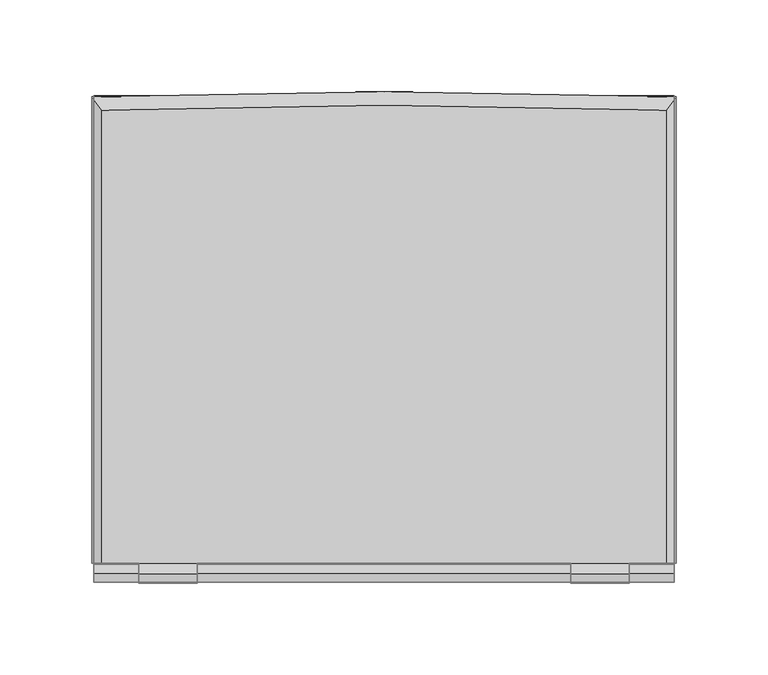
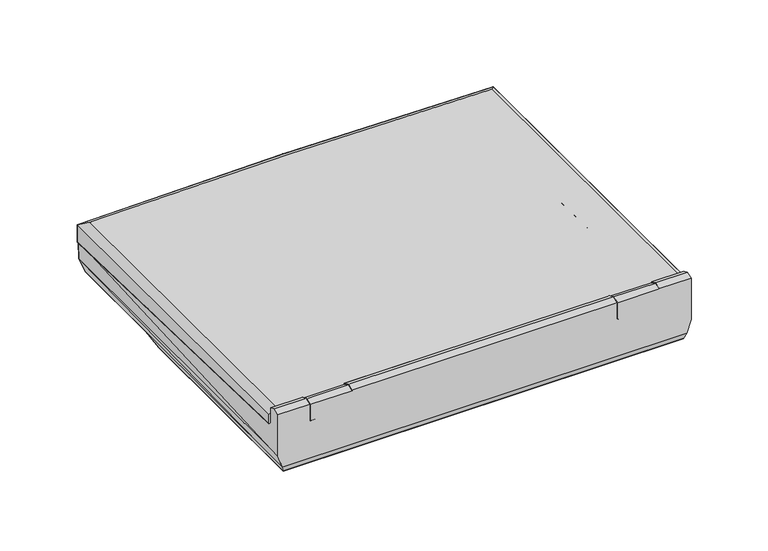
"""IFC4 building model written with IfcOpenShell, lengths in millimetres: proxy geometry."""

from ifc_helpers import new_model, si_unit, origin, place, context, project, spatial, triangles, source, transform, mapped, element, save


def entourage_d5009a78(model_context):
    return source(origin(), model_context, "Body", "Tessellation", [
        triangles([(158.4296465, 167.58125, 28.2218852), (101.7496669, -97.7313892, 35.1332116), (101.7496669, -97.7313892, 48.4910445), (101.7496669, -92.7961799, 50.2665039), (101.7496669, -87.9168539, 48.183705), (101.7496669, -87.9168539, 35.1332116), (158.4296465, -87.9168539, 35.1332116), (133.8221823, -97.7288549, 35.1332116), (133.8221823, -97.7313892, 48.4910445), (133.8221823, -92.7961799, 50.2665039), (133.8221823, -87.9168539, 48.183705), (133.8221823, -87.9168539, 35.1332116), (-158.4321899, 167.58125, 28.2218852), (-101.7496669, -97.7313892, 35.1332116), (-101.7496669, -97.7313892, 48.4910445), (-101.7496669, -92.7961799, 50.2665039), (-101.7496669, -87.9168539, 48.183705), (-101.7496669, -87.9168539, 35.1332116), (-85.2320795, 66.8399699, 31.8083578), (144.8813183, 53.1646373, 31.9658382), (-85.2320795, 53.1646373, 31.9658382), (144.8813183, -60.6703247, 34.190875), (-146.9209376, -74.3380361, 34.2924744), (-146.9209376, 66.8399699, 31.8083578), (-158.4321899, -87.9168539, 35.1332116), (-133.8247257, -97.7313892, 35.1332116), (-133.8247257, -97.7313892, 48.4910445), (-133.8247257, -92.7961799, 50.2665039), (-133.8247257, -87.9168539, 48.183705), (-133.8247257, -87.9168539, 35.1332116), (142.7070869, -58.4935454, 29.3902823), (-15.8851291, -74.3380361, 34.2924744), (-19.0347234, -72.5752803, 29.491884), (-15.8851291, -60.6703247, 34.190875), (-19.0347234, -58.4935454, 29.3902823), (155.2851437, 164.0506697, 4.7853507), (155.2851437, 83.3296157, 4.8691705), (153.4715916, 69.0040457, 0.0), (153.4715916, -95.8771965, 0.0), (-155.2876871, 164.0506697, 4.7853507), (-155.2851437, 83.3296157, 4.8691705), (-153.4715916, 69.0040457, 0.0), (-153.4715916, -95.8771965, 0.0), (155.2851437, -97.7313892, 4.8691705), (158.4296465, -97.7313892, 14.9046918), (158.4296465, -97.7313892, 48.4910445), (-155.2851437, -97.7313892, 4.8691705), (-158.4321899, -97.7313892, 14.9046918), (-158.4321899, -97.7313892, 48.4910445), (158.4296465, -92.7961799, 50.2665039), (158.4296465, -87.9168539, 48.183705), (-158.4321899, -92.7961799, 50.2665039), (-158.4321899, -87.9168539, 48.183705), (158.6201509, 166.809095, 14.9046918), (-158.6201509, 166.809095, 14.9046918), (-87.4063109, 64.9654568, 27.0992089), (142.7070869, 51.2901197, 27.2541481), (-87.4063109, 51.2901197, 27.2541481), (-144.7466972, -72.5752803, 29.491884), (-144.7466972, 64.9654568, 27.0992089), (-141.2262725, 62.1181197, 32.971677), (-90.9267446, 62.1181197, 32.971677), (138.3738576, 48.4427871, 33.1266163), (-90.9267446, 48.4427871, 33.1266163), (138.3738576, -55.455713, 35.1128913), (-141.2262725, -69.5374479, 35.2170319), (-21.8820582, -55.455713, 35.1128913), (-21.8820582, -69.5374479, 35.2170319), (0.0, -78.9883291, 38.7773705), (0.0, 148.3190173, 34.6998669), (145.6915795, -78.989728, 38.772488), (145.6915795, 148.3190173, 34.6998669), (-145.1099199, -78.989728, 38.772488), (-145.1099199, 148.3190173, 34.6998669), (0.0, -80.5417862, 35.3042041), (0.0, 149.5301715, 31.5516783), (147.9064516, -80.5407416, 35.2986198), (147.9064516, 149.5301715, 31.5516783), (-147.324792, -80.5407416, 35.2986198), (-147.324792, 149.5301715, 31.5516783), (0.0, 169.8360542, 28.0754711), (0.0, 169.7931244, 42.3380044), (159.4431202, 167.0172945, 28.4001878), (159.4431202, 166.9750551, 42.6651601), (-159.4431202, 167.0172945, 28.4001878), (-159.4431202, 166.9750551, 42.6651601), (0.0, 162.5079949, 46.5302948), (0.0, -87.4703786, 47.1442881), (101.7496669, -98.2048796, 48.5682428), (154.0176883, 159.6892353, 46.8550116), (101.7496669, -87.4703786, 47.1442881), (133.8221823, -98.2034898, 48.5546353), (133.7332797, -87.4703786, 47.1442881), (154.0176883, -87.4703786, 47.1442881), (133.8221823, -93.2694705, 50.3265066), (101.7496669, -93.2694705, 50.3265066), (159.4431202, -87.4719137, 42.9645241), (-101.7496669, -98.2048796, 48.5682428), (-154.0176883, 159.6892353, 46.8550116), (-101.7496669, -87.4703786, 47.1442881), (-133.8221823, -98.2034898, 48.5546353), (-133.7332797, -87.4703786, 47.1442881), (-154.0176883, -87.4703786, 47.1442881), (-133.8221823, -93.2694705, 50.3265066), (-101.7496669, -93.2694705, 50.3265066), (-159.4431202, -87.4719137, 42.9645241), (0.0, -87.4749386, 35.3976872), (101.7496669, -98.2071505, 35.198576), (101.7496669, -87.4735397, 35.4025697), (133.8221823, -98.2071505, 35.198576), (-101.7496669, -98.2071505, 35.198576), (-101.7496669, -87.4735397, 35.4025697), (-133.8221823, -98.2071505, 35.198576), (133.7332797, -87.4735397, 35.4025697), (159.4431202, -87.4732036, 35.3945442), (-133.7332797, -87.4735397, 35.4025697), (-159.4431202, -87.4732036, 35.3945442), (0.0, 167.5662254, 28.1582286), (156.9437634, 164.7481562, 28.4853866), (159.4431202, 69.7213075, 31.0754356), (0.0, 165.6878881, 31.2097115), (155.5010462, 162.8722532, 31.5361701), (-156.9437634, 164.7481562, 28.4853866), (-159.4431202, 69.7213075, 31.0754356), (-155.5010462, 162.8722532, 31.5361701)], [[19, 1, 13], [2, 6, 3], [3, 6, 4], [4, 6, 5], [12, 6, 8], [8, 6, 2], [11, 12, 10], [10, 12, 9], [9, 12, 8], [21, 20, 19], [20, 1, 19], [22, 6, 12], [1, 20, 7], [22, 12, 7], [23, 6, 32], [18, 6, 23], [19, 13, 24], [14, 15, 18], [15, 16, 18], [16, 17, 18], [30, 26, 18], [26, 14, 18], [29, 28, 30], [28, 27, 30], [27, 26, 30], [24, 25, 23], [23, 30, 18], [13, 25, 24], [23, 25, 30], [32, 6, 22], [22, 34, 32], [31, 33, 35], [37, 41, 36], [36, 41, 40], [42, 41, 38], [38, 41, 37], [39, 43, 38], [38, 43, 42], [44, 8, 2], [8, 44, 45], [45, 46, 9], [9, 8, 45], [44, 47, 39], [39, 47, 43], [2, 14, 47], [2, 47, 44], [3, 15, 14], [3, 14, 2], [47, 14, 26], [26, 48, 47], [48, 27, 49], [27, 48, 26], [50, 51, 11], [11, 10, 50], [5, 17, 16], [5, 16, 4], [52, 29, 53], [29, 52, 28], [46, 50, 10], [10, 9, 46], [4, 16, 15], [4, 15, 3], [49, 28, 52], [28, 49, 27], [13, 1, 55], [55, 1, 54], [55, 54, 40], [40, 54, 36], [55, 40, 41], [48, 52, 25], [52, 48, 49], [53, 25, 52], [41, 43, 47], [13, 48, 25], [55, 47, 48], [43, 41, 42], [48, 13, 55], [47, 55, 41], [51, 7, 12], [12, 11, 51], [6, 18, 17], [6, 17, 5], [53, 30, 25], [30, 53, 29], [54, 37, 36], [45, 7, 50], [50, 46, 45], [51, 50, 7], [37, 44, 39], [1, 7, 45], [54, 45, 44], [39, 38, 37], [45, 54, 1], [44, 37, 54], [57, 31, 22], [23, 32, 33], [33, 59, 23], [20, 21, 58], [58, 57, 20], [21, 19, 56], [56, 58, 21], [19, 24, 60], [60, 56, 19], [24, 23, 59], [59, 60, 24], [34, 22, 31], [31, 35, 34], [33, 32, 34], [34, 35, 33], [59, 35, 33], [20, 22, 7], [22, 20, 57], [67, 65, 63], [67, 63, 64], [64, 62, 61], [66, 64, 61], [31, 57, 63], [63, 65, 31], [35, 31, 65], [65, 67, 35], [57, 58, 64], [64, 63, 57], [58, 56, 62], [62, 64, 58], [56, 60, 61], [61, 62, 56], [60, 59, 66], [66, 61, 60], [66, 67, 64], [68, 66, 59], [59, 33, 68], [35, 67, 68], [68, 33, 35], [66, 68, 67], [69, 70, 72], [69, 72, 71], [69, 74, 70], [69, 73, 74], [76, 78, 72], [72, 70, 76], [77, 75, 69], [69, 71, 77], [78, 77, 71], [71, 72, 78], [76, 74, 80], [74, 76, 70], [79, 69, 75], [69, 79, 73], [80, 73, 79], [73, 80, 74], [81, 82, 84], [81, 84, 83], [81, 86, 82], [81, 85, 86], [82, 87, 90], [82, 90, 84], [87, 88, 91], [87, 91, 90], [90, 91, 93], [96, 89, 92], [96, 92, 95], [90, 93, 94], [97, 90, 94], [91, 95, 93], [91, 96, 95], [97, 84, 90], [82, 99, 87], [82, 86, 99], [87, 100, 88], [87, 99, 100], [99, 102, 100], [105, 101, 98], [105, 104, 101], [102, 99, 103], [106, 103, 99], [100, 102, 104], [100, 104, 105], [106, 99, 86], [89, 108, 110], [89, 110, 92], [96, 91, 89], [89, 91, 108], [108, 91, 109], [91, 88, 109], [109, 88, 107], [98, 113, 111], [98, 101, 113], [105, 98, 100], [98, 111, 100], [111, 112, 100], [100, 112, 88], [112, 107, 88], [93, 114, 115], [93, 115, 97], [95, 92, 93], [93, 92, 114], [114, 92, 110], [93, 97, 94], [102, 117, 116], [102, 106, 117], [104, 102, 101], [102, 116, 101], [116, 113, 101], [102, 103, 106], [108, 109, 114], [108, 114, 110], [81, 83, 119], [109, 107, 75], [75, 77, 109], [114, 109, 77], [120, 115, 77], [114, 77, 115], [119, 118, 81], [77, 78, 120], [119, 120, 122], [76, 121, 122], [76, 122, 78], [119, 122, 121], [119, 121, 118], [120, 78, 122], [83, 120, 119], [111, 116, 112], [111, 113, 116], [81, 123, 85], [112, 75, 107], [75, 112, 79], [116, 79, 112], [124, 79, 117], [117, 79, 116], [123, 81, 118], [79, 124, 80], [123, 125, 124], [76, 125, 121], [76, 80, 125], [123, 121, 125], [123, 118, 121], [124, 125, 80], [85, 123, 124], [117, 86, 124], [117, 106, 86], [124, 86, 85], [115, 120, 84], [115, 84, 97], [120, 83, 84]], closed=False),
    ])


if __name__ == "__main__":
    model = new_model("IFC4")
    model_context = context("Model", 3, world=origin())
    ifc_project = project(units=[si_unit("LENGTHUNIT", "METRE", prefix="MILLI")], contexts=[model_context])
    site = spatial("IfcSite", under=ifc_project)
    building = spatial("IfcBuilding", under=site)
    placement = place(None, origin())
    entourage_shape = entourage_d5009a78(model_context)
    element("IfcBuildingElementProxy", 1, Name="Entourage", at=placement, inside=building, context=model_context, shape_type="MappedRepresentation", body=[
        mapped(entourage_shape, transform((0.0, 0.0, 0.0), x_axis=(1.0, 0.0, 0.0), y_axis=(0.0, 1.0, 0.0), z_axis=(0.0, 0.0, 1.0))),
    ])
    save(model, "model.ifc")

# Revit data of these elements
# Type
#   built-in parameter 1005198 = "{2, 15},{39, RPC-16-N04H-AQSP-D1N4-43SU-6GKQ-C3KU-1C},{1, 0},{1, 0},{2, 41},{1, 8},{5, Color},{1, 0},{1, 0},{3, 0.8},{3, 0.8},{3, 0.8},{1, 8},{7, BBoxMin},{1, 0},{1, 0},{1, 0},{1, 0},{1, 0},{1, 8},{7, BBoxMax},{1, 0},{1, 0},{1, 0},{1, 0},{1, 0},{2, 11},{9, RPCTypeId},{1, 0},{1, 0},{39, RPC-16-N04H-AQSP-D1N4-43SU-6GKQ-C3KU-1C},{1, 6},{14, RPCPlantHeight},{1, 0},{1, 0},{7, 2.28517},{2, 11},{7, keyword},{1, 0},{1, 0},{31, :Geometry:RPC:Notebook Computer},{2, 11},{8, category},{1, 0},{1, 0},{15, :Office Clutter},{2, 11},{12, LocalizedUID},{1, 0},{1, 0},{17, Notebook Computer},{2, 14},{6, Height},{1, 0},{1, 0},{7, 2.28517},{1, 2},{16, Cast Reflections},{1, 0},{1, 0},{1, 0},{1, 4},{4, Open},{1, 0},{1, 0},{4, -106},{1, 2},{5, Power},{1, 0},{1, 0},{1, 1},{2, 11},{14, Screen Preview},{1, 0},{1, 0},{70, __RPC:/object data/textures/object/Top/TopScreen/textures/on/rgb/0/0/0},{2, 11},{16, i_Screen Preview},{1, 0},{1, 0},{0, },{1, 2},{13, Custom Screen},{1, 0},{1, 0},{1, 0},{2, 11},{16, Screen File Name},{1, 0},{1, 0},{0, },{2, 11},{20, AdvancedUIDefinition},{1, 0},{1, 0},{0, },{2, 11},{10, AssetLibID},{1, 0},{1, 0},{36, 4D3F6E72-3F99-4203-98E9-AF80B3C7A7A4},{2, 11},{10, BaseSchema},{1, 0},{1, 0},{9, RPCSchema},{2, 11},{12, ExchangeGUID},{1, 0},{1, 0},{0, },{1, 2},{6, Hidden},{1, 0},{1, 0},{1, 0},{1, 4},{11, RPCCategory},{1, 0},{1, 0},{1, 0},{2, 11},{8, RPCImage},{1, 0},{1, 0},{0, },{1, 4},{13, SchemaVersion},{1, 0},{1, 0},{1, 4},{2, 11},{12, UIDefinition},{1, 0},{1, 0},{0, },{2, 11},{6, UIName},{1, 0},{1, 0},{39, RPC-16-N04H-AQSP-D1N4-43SU-6GKQ-C3KU-1C},{2, 11},{11, VersionGUID},{1, 0},{1, 0},{9, RPCSchema},{2, 11},{9, assettype},{1, 0},{1, 0},{11, RPCGeometry},{2, 11},{11, description},{1, 0},{1, 0},{0, },{2, 11},{9, localname},{1, 0},{1, 0},{3, RPC},{2, 11},{9, localtype},{1, 0},{1, 0},{3, RPC},{1, 4},{8, revision},{1, 0},{1, 0},{1, 1},{2, 11},{9, thumbnail},{1, 0},{1, 0},{0, },{1, 4},{7, version},{1, 0},{1, 0},{1, 1},{1, 2},{20, RPC_Cast Reflections},{1, 0},{1, 0},{1, 1},{1, 4},{8, RPC_Open},{1, 0},{1, 0},{4, -106},{1, 2},{9, RPC_Power},{1, 0},{1, 0},{1, 1},{2, 11},{18, RPC_Screen Preview},{1, 0},{1, 0},{70, __RPC:/object data/textures/object/Top/TopScreen/textures/on/rgb/0/0/0},{2, 11},{20, RPC_i_Screen Preview},{1, 0},{1, 0},{0, },{1, 2},{17, RPC_Custom Screen},{1, 0},{1, 0},{1, 0},{2, 11},{20, RPC_Screen File Name},{1, 0},{1, 0},{0, },{21, assetlibrary_base.fbx},{1, 5},"
#   built-in parameter 1005195 = "RPC-16-N04H-AQSP-D1N4-43SU-6GKQ-C3KU-1C"
#   Height = 0
